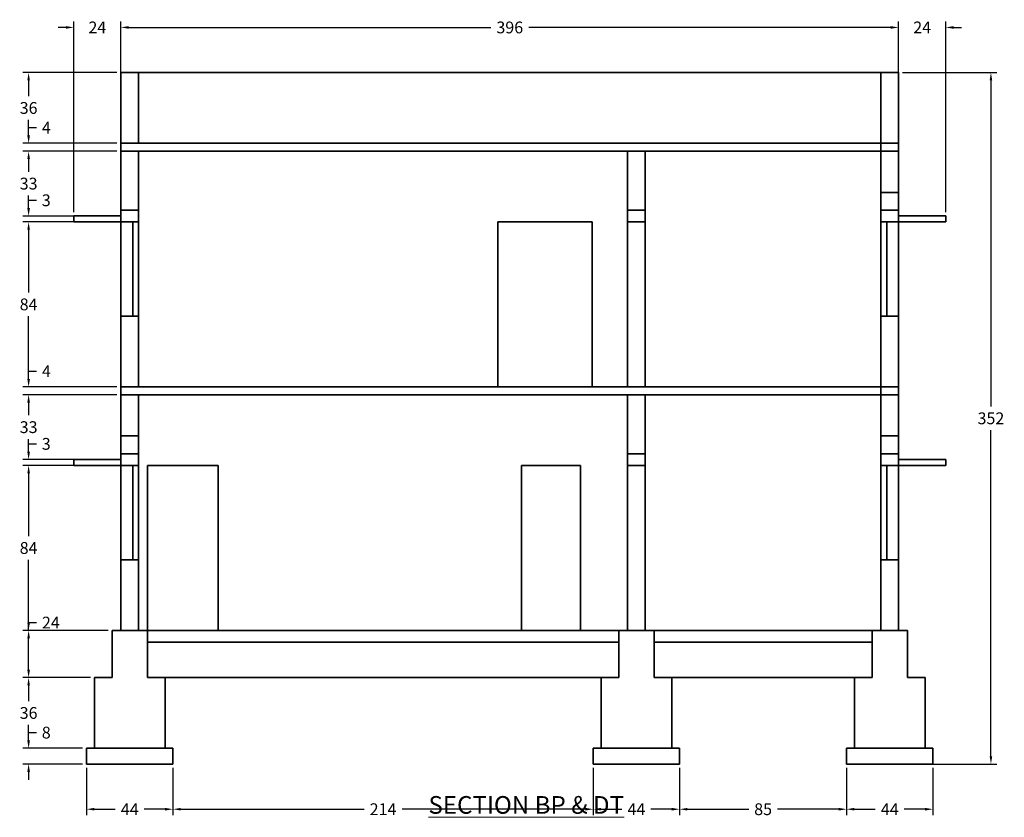
# Model space of a CAD drawing. Units: inches. Extents: x 853 to 2068, y 1026 to 2097.
# Tile 6 of 6: x 1529 to 2030, y 1690 to 2096. Entities that reach past the tile are written whole.
import ezdxf

# ---------------------------------------------------------------- set-up
doc = ezdxf.new("R2010")
doc.units = ezdxf.units.IN
doc.header["$MEASUREMENT"] = 0
for name, color, linetype, lineweight in [('A-ANNO-DIMS', 2, 'Continuous', 18), ('A-ANNO-TEXT', 3, 'Continuous', 18), ('A-SECT', 1, 'Continuous', 35)]:
    doc.layers.add(name, color=color, linetype=linetype, lineweight=lineweight)
doc.styles.get("Standard").update_dxf_attribs({"font": 'arial.ttf'})
doc.dimstyles.get("Standard").update_dxf_attribs({"dimtxt": 6, "dimasz": 4, "dimexe": 3, "dimexo": 2, "dimgap": 3, "dimtad": 0, "dimtih": 1, "dimtoh": 1, "dimdec": 0, "dimzin": 0, "dimdsep": 46, "dimlunit": 3, "dimtxsty": 'Standard', "dimcen": 3, "dimadec": 0, "dimazin": 0, "dimtfac": 1, "dimtdec": 0, "dimtofl": 0, "dimtmove": 0, "dimatfit": 3, "dimfxl": 1, "dimtolj": 1, "dimtzin": 0, "dimarcsym": 0})

# ---------------------------------------------------------------- blocks, each defined once
blk = doc.blocks.new('*D94')
at = {"layer": 'A-ANNO-DIMS', "color": 0, "lineweight": -2, "transparency": 16777216}
for p, q in [((1533.64, 1729.25), (1533.64, 1733.25)), ((1533.64, 1733.25), (1537.64, 1733.25)), ((1561.14, 1725.25), (1530.64, 1725.25)), ((1561.14, 1717.25), (1530.64, 1717.25)), ((1533.64, 1713.25), (1533.64, 1709.25))]:
    blk.add_line(p, q, dxfattribs=at)
at = {"layer": 'A-ANNO-DIMS', "color": 0, "transparency": 16777216}
for points in [[(1532.98, 1729.25), (1534.31, 1729.25), (1533.64, 1725.25)], [(1532.98, 1713.25), (1534.31, 1713.25), (1533.64, 1717.25)]]:
    blk.add_solid(points, dxfattribs=at)
at = {"layer": 'Defpoints', "color": 0, "transparency": 16777216}
for p in [(1533.64, 1725.25), (1563.14, 1725.25), (1563.14, 1717.25)]:
    blk.add_point(p, dxfattribs=at)
at = {"layer": 'A-ANNO-DIMS', "color": 0, "transparency": 16777216, "insert": (1542.62, 1733.25), "char_height": 6, "attachment_point": 5}
blk.add_mtext('\\A1;8', dxfattribs=at)
blk = doc.blocks.new('*D95')
at = {"layer": 'A-ANNO-DIMS', "color": 0, "lineweight": -2, "transparency": 16777216}
for p, q in [((1565.14, 1761.25), (1530.64, 1761.25)), ((1533.64, 1757.25), (1533.64, 1749.32)), ((1533.64, 1729.25), (1533.64, 1737.19)), ((1561.14, 1725.25), (1530.64, 1725.25))]:
    blk.add_line(p, q, dxfattribs=at)
at = {"layer": 'A-ANNO-DIMS', "color": 0, "transparency": 16777216}
for points in [[(1532.98, 1757.25), (1534.31, 1757.25), (1533.64, 1761.25)], [(1532.98, 1729.25), (1534.31, 1729.25), (1533.64, 1725.25)]]:
    blk.add_solid(points, dxfattribs=at)
at = {"layer": 'Defpoints', "color": 0, "transparency": 16777216}
for p in [(1533.64, 1761.25), (1567.14, 1761.25), (1563.14, 1725.25)]:
    blk.add_point(p, dxfattribs=at)
at = {"layer": 'A-ANNO-DIMS', "color": 0, "transparency": 16777216, "insert": (1533.64, 1743.25), "char_height": 6, "attachment_point": 5}
blk.add_mtext('\\A1;36', dxfattribs=at)
blk = doc.blocks.new('*D96')
at = {"layer": 'A-ANNO-DIMS', "color": 0, "lineweight": -2, "transparency": 16777216}
for p, q in [((1574.14, 1785.25), (1530.64, 1785.25)), ((1533.64, 1785.25), (1533.64, 1789.25)), ((1533.64, 1789.25), (1537.64, 1789.25)), ((1533.64, 1765.25), (1533.64, 1781.25)), ((1565.14, 1761.25), (1530.64, 1761.25))]:
    blk.add_line(p, q, dxfattribs=at)
at = {"layer": 'A-ANNO-DIMS', "color": 0, "transparency": 16777216}
for points in [[(1532.98, 1781.25), (1534.31, 1781.25), (1533.64, 1785.25)], [(1532.98, 1765.25), (1534.31, 1765.25), (1533.64, 1761.25)]]:
    blk.add_solid(points, dxfattribs=at)
at = {"layer": 'Defpoints', "color": 0, "transparency": 16777216}
for p in [(1533.64, 1785.25), (1576.14, 1785.25), (1567.14, 1761.25)]:
    blk.add_point(p, dxfattribs=at)
at = {"layer": 'A-ANNO-DIMS', "color": 0, "transparency": 16777216, "insert": (1544.98, 1789.25), "char_height": 6, "attachment_point": 5}
blk.add_mtext('\\A1;24', dxfattribs=at)
blk = doc.blocks.new('*D97')
at = {"layer": 'A-ANNO-DIMS', "color": 0, "lineweight": -2, "transparency": 16777216}
for p, q in [((1578.64, 1869.25), (1530.64, 1869.25)), ((1533.64, 1865.25), (1533.64, 1833.31)), ((1533.64, 1789.25), (1533.64, 1821.19)), ((1574.14, 1785.25), (1530.64, 1785.25))]:
    blk.add_line(p, q, dxfattribs=at)
at = {"layer": 'A-ANNO-DIMS', "color": 0, "transparency": 16777216}
for points in [[(1532.98, 1865.25), (1534.31, 1865.25), (1533.64, 1869.25)], [(1532.98, 1789.25), (1534.31, 1789.25), (1533.64, 1785.25)]]:
    blk.add_solid(points, dxfattribs=at)
at = {"layer": 'Defpoints', "color": 0, "transparency": 16777216}
for p in [(1533.64, 1869.25), (1580.64, 1869.25), (1576.14, 1785.25)]:
    blk.add_point(p, dxfattribs=at)
at = {"layer": 'A-ANNO-DIMS', "color": 0, "transparency": 16777216, "insert": (1533.64, 1827.25), "char_height": 6, "attachment_point": 5}
blk.add_mtext('\\A1;84', dxfattribs=at)
blk = doc.blocks.new('*D98')
at = {"layer": 'A-ANNO-DIMS', "color": 0, "lineweight": -2, "transparency": 16777216}
for p, q in [((1533.64, 1876.25), (1533.64, 1880.25)), ((1533.64, 1880.25), (1537.64, 1880.25)), ((1578.64, 1872.25), (1530.64, 1872.25)), ((1578.64, 1869.25), (1530.64, 1869.25)), ((1533.64, 1865.25), (1533.64, 1861.25))]:
    blk.add_line(p, q, dxfattribs=at)
at = {"layer": 'A-ANNO-DIMS', "color": 0, "transparency": 16777216}
for points in [[(1532.98, 1876.25), (1534.31, 1876.25), (1533.64, 1872.25)], [(1532.98, 1865.25), (1534.31, 1865.25), (1533.64, 1869.25)]]:
    blk.add_solid(points, dxfattribs=at)
at = {"layer": 'Defpoints', "color": 0, "transparency": 16777216}
for p in [(1533.64, 1872.25), (1580.64, 1872.25), (1580.64, 1869.25)]:
    blk.add_point(p, dxfattribs=at)
at = {"layer": 'A-ANNO-DIMS', "color": 0, "transparency": 16777216, "insert": (1542.61, 1880.25), "char_height": 6, "attachment_point": 5}
blk.add_mtext('\\A1;3', dxfattribs=at)
blk = doc.blocks.new('*D99')
at = {"layer": 'A-ANNO-DIMS', "color": 0, "lineweight": -2, "transparency": 16777216}
for p, q in [((1578.64, 1905.25), (1530.64, 1905.25)), ((1533.64, 1901.25), (1533.64, 1894.82)), ((1533.64, 1876.25), (1533.64, 1882.69)), ((1578.64, 1872.25), (1530.64, 1872.25))]:
    blk.add_line(p, q, dxfattribs=at)
at = {"layer": 'A-ANNO-DIMS', "color": 0, "transparency": 16777216}
for points in [[(1532.98, 1901.25), (1534.31, 1901.25), (1533.64, 1905.25)], [(1532.98, 1876.25), (1534.31, 1876.25), (1533.64, 1872.25)]]:
    blk.add_solid(points, dxfattribs=at)
at = {"layer": 'Defpoints', "color": 0, "transparency": 16777216}
for p in [(1533.64, 1905.25), (1580.64, 1905.25), (1580.64, 1872.25)]:
    blk.add_point(p, dxfattribs=at)
at = {"layer": 'A-ANNO-DIMS', "color": 0, "transparency": 16777216, "insert": (1533.64, 1888.75), "char_height": 6, "attachment_point": 5}
blk.add_mtext('\\A1;33', dxfattribs=at)
blk = doc.blocks.new('*D100')
at = {"layer": 'A-ANNO-DIMS', "color": 0, "lineweight": -2, "transparency": 16777216}
for p, q in [((1533.64, 1913.25), (1533.64, 1917.25)), ((1533.64, 1917.25), (1537.64, 1917.25)), ((1578.64, 1909.25), (1530.64, 1909.25)), ((1578.64, 1905.25), (1530.64, 1905.25)), ((1533.64, 1901.25), (1533.64, 1897.25))]:
    blk.add_line(p, q, dxfattribs=at)
at = {"layer": 'A-ANNO-DIMS', "color": 0, "transparency": 16777216}
for points in [[(1532.98, 1913.25), (1534.31, 1913.25), (1533.64, 1909.25)], [(1532.98, 1901.25), (1534.31, 1901.25), (1533.64, 1905.25)]]:
    blk.add_solid(points, dxfattribs=at)
at = {"layer": 'Defpoints', "color": 0, "transparency": 16777216}
for p in [(1533.64, 1909.25), (1580.64, 1909.25), (1580.64, 1905.25)]:
    blk.add_point(p, dxfattribs=at)
at = {"layer": 'A-ANNO-DIMS', "color": 0, "transparency": 16777216, "insert": (1542.72, 1917.25), "char_height": 6, "attachment_point": 5}
blk.add_mtext('\\A1;4', dxfattribs=at)
blk = doc.blocks.new('*D101')
at = {"layer": 'A-ANNO-DIMS', "color": 0, "lineweight": -2, "transparency": 16777216}
for p, q in [((1578.64, 1993.25), (1530.64, 1993.25)), ((1533.64, 1989.25), (1533.64, 1957.31)), ((1533.64, 1913.25), (1533.64, 1945.19)), ((1578.64, 1909.25), (1530.64, 1909.25))]:
    blk.add_line(p, q, dxfattribs=at)
at = {"layer": 'A-ANNO-DIMS', "color": 0, "transparency": 16777216}
for points in [[(1532.98, 1989.25), (1534.31, 1989.25), (1533.64, 1993.25)], [(1532.98, 1913.25), (1534.31, 1913.25), (1533.64, 1909.25)]]:
    blk.add_solid(points, dxfattribs=at)
at = {"layer": 'Defpoints', "color": 0, "transparency": 16777216}
for p in [(1533.64, 1993.25), (1580.64, 1993.25), (1580.64, 1909.25)]:
    blk.add_point(p, dxfattribs=at)
at = {"layer": 'A-ANNO-DIMS', "color": 0, "transparency": 16777216, "insert": (1533.64, 1951.25), "char_height": 6, "attachment_point": 5}
blk.add_mtext('\\A1;84', dxfattribs=at)
blk = doc.blocks.new('*D102')
at = {"layer": 'A-ANNO-DIMS', "color": 0, "lineweight": -2, "transparency": 16777216}
for p, q in [((1533.64, 2000.25), (1533.64, 2004.25)), ((1533.64, 2004.25), (1537.64, 2004.25)), ((1578.64, 1996.25), (1530.64, 1996.25)), ((1578.64, 1993.25), (1530.64, 1993.25)), ((1533.64, 1989.25), (1533.64, 1985.25))]:
    blk.add_line(p, q, dxfattribs=at)
at = {"layer": 'A-ANNO-DIMS', "color": 0, "transparency": 16777216}
for points in [[(1532.98, 2000.25), (1534.31, 2000.25), (1533.64, 1996.25)], [(1532.98, 1989.25), (1534.31, 1989.25), (1533.64, 1993.25)]]:
    blk.add_solid(points, dxfattribs=at)
at = {"layer": 'Defpoints', "color": 0, "transparency": 16777216}
for p in [(1533.64, 1996.25), (1580.64, 1996.25), (1580.64, 1993.25)]:
    blk.add_point(p, dxfattribs=at)
at = {"layer": 'A-ANNO-DIMS', "color": 0, "transparency": 16777216, "insert": (1542.61, 2004.25), "char_height": 6, "attachment_point": 5}
blk.add_mtext('\\A1;3', dxfattribs=at)
blk = doc.blocks.new('*D103')
at = {"layer": 'A-ANNO-DIMS', "color": 0, "lineweight": -2, "transparency": 16777216}
for p, q in [((1578.64, 2029.25), (1530.64, 2029.25)), ((1533.64, 2025.25), (1533.64, 2018.82)), ((1533.64, 2000.25), (1533.64, 2006.69)), ((1578.64, 1996.25), (1530.64, 1996.25))]:
    blk.add_line(p, q, dxfattribs=at)
at = {"layer": 'A-ANNO-DIMS', "color": 0, "transparency": 16777216}
for points in [[(1532.98, 2025.25), (1534.31, 2025.25), (1533.64, 2029.25)], [(1532.98, 2000.25), (1534.31, 2000.25), (1533.64, 1996.25)]]:
    blk.add_solid(points, dxfattribs=at)
at = {"layer": 'Defpoints', "color": 0, "transparency": 16777216}
for p in [(1533.64, 2029.25), (1580.64, 2029.25), (1580.64, 1996.25)]:
    blk.add_point(p, dxfattribs=at)
at = {"layer": 'A-ANNO-DIMS', "color": 0, "transparency": 16777216, "insert": (1533.64, 2012.75), "char_height": 6, "attachment_point": 5}
blk.add_mtext('\\A1;33', dxfattribs=at)
blk = doc.blocks.new('*D104')
at = {"layer": 'A-ANNO-DIMS', "color": 0, "lineweight": -2, "transparency": 16777216}
for p, q in [((1533.64, 2037.25), (1533.64, 2041.25)), ((1533.64, 2041.25), (1537.64, 2041.25)), ((1578.64, 2033.25), (1530.64, 2033.25)), ((1578.64, 2029.25), (1530.64, 2029.25)), ((1533.64, 2025.25), (1533.64, 2021.25))]:
    blk.add_line(p, q, dxfattribs=at)
at = {"layer": 'A-ANNO-DIMS', "color": 0, "transparency": 16777216}
for points in [[(1532.98, 2037.25), (1534.31, 2037.25), (1533.64, 2033.25)], [(1532.98, 2025.25), (1534.31, 2025.25), (1533.64, 2029.25)]]:
    blk.add_solid(points, dxfattribs=at)
at = {"layer": 'Defpoints', "color": 0, "transparency": 16777216}
for p in [(1533.64, 2033.25), (1580.64, 2033.25), (1580.64, 2029.25)]:
    blk.add_point(p, dxfattribs=at)
at = {"layer": 'A-ANNO-DIMS', "color": 0, "transparency": 16777216, "insert": (1542.72, 2041.25), "char_height": 6, "attachment_point": 5}
blk.add_mtext('\\A1;4', dxfattribs=at)
blk = doc.blocks.new('*D105')
at = {"layer": 'A-ANNO-DIMS', "color": 0, "lineweight": -2, "transparency": 16777216}
for p, q in [((1578.64, 2069.25), (1530.64, 2069.25)), ((1533.64, 2065.25), (1533.64, 2057.32)), ((1533.64, 2037.25), (1533.64, 2045.19)), ((1578.64, 2033.25), (1530.64, 2033.25))]:
    blk.add_line(p, q, dxfattribs=at)
at = {"layer": 'A-ANNO-DIMS', "color": 0, "transparency": 16777216}
for points in [[(1532.98, 2065.25), (1534.31, 2065.25), (1533.64, 2069.25)], [(1532.98, 2037.25), (1534.31, 2037.25), (1533.64, 2033.25)]]:
    blk.add_solid(points, dxfattribs=at)
at = {"layer": 'Defpoints', "color": 0, "transparency": 16777216}
for p in [(1533.64, 2069.25), (1580.64, 2069.25), (1580.64, 2033.25)]:
    blk.add_point(p, dxfattribs=at)
at = {"layer": 'A-ANNO-DIMS', "color": 0, "transparency": 16777216, "insert": (1533.64, 2051.25), "char_height": 6, "attachment_point": 5}
blk.add_mtext('\\A1;36', dxfattribs=at)
blk = doc.blocks.new('*D106')
at = {"layer": 'A-ANNO-DIMS', "color": 0, "lineweight": -2, "transparency": 16777216}
for p, q in [((1978.64, 2069.25), (2026.64, 2069.25)), ((2023.64, 2065.25), (2023.64, 1899.32)), ((2023.64, 1721.25), (2023.64, 1887.19)), ((1969.64, 1717.25), (2026.64, 1717.25))]:
    blk.add_line(p, q, dxfattribs=at)
at = {"layer": 'A-ANNO-DIMS', "color": 0, "transparency": 16777216}
for points in [[(2022.98, 2065.25), (2024.31, 2065.25), (2023.64, 2069.25)], [(2022.98, 1721.25), (2024.31, 1721.25), (2023.64, 1717.25)]]:
    blk.add_solid(points, dxfattribs=at)
at = {"layer": 'Defpoints', "color": 0, "transparency": 16777216}
for p in [(1976.64, 2069.25), (2023.64, 2069.25), (1967.64, 1717.25)]:
    blk.add_point(p, dxfattribs=at)
at = {"layer": 'A-ANNO-DIMS', "color": 0, "transparency": 16777216, "insert": (2023.64, 1893.25), "char_height": 6, "attachment_point": 5}
blk.add_mtext('\\A1;352', dxfattribs=at)
blk = doc.blocks.new('*D107')
at = {"layer": 'A-ANNO-DIMS', "color": 0, "lineweight": -2, "transparency": 16777216}
for p, q in [((1563.14, 1715.25), (1563.14, 1691.25)), ((1607.14, 1715.25), (1607.14, 1691.25)), ((1567.14, 1694.25), (1577.74, 1694.25)), ((1603.14, 1694.25), (1592.55, 1694.25))]:
    blk.add_line(p, q, dxfattribs=at)
at = {"layer": 'A-ANNO-DIMS', "color": 0, "transparency": 16777216}
for points in [[(1567.14, 1694.92), (1567.14, 1693.58), (1563.14, 1694.25)], [(1603.14, 1694.92), (1603.14, 1693.58), (1607.14, 1694.25)]]:
    blk.add_solid(points, dxfattribs=at)
at = {"layer": 'Defpoints', "color": 0, "transparency": 16777216}
for p in [(1563.14, 1717.25), (1607.14, 1717.25), (1607.14, 1694.25)]:
    blk.add_point(p, dxfattribs=at)
at = {"layer": 'A-ANNO-DIMS', "color": 0, "transparency": 16777216, "insert": (1585.14, 1694.25), "char_height": 6, "attachment_point": 5}
blk.add_mtext('\\A1;44', dxfattribs=at)
blk = doc.blocks.new('*D108')
at = {"layer": 'A-ANNO-DIMS', "color": 0, "lineweight": -2, "transparency": 16777216}
for p, q in [((1607.14, 1715.25), (1607.14, 1691.25)), ((1821.14, 1715.25), (1821.14, 1691.25)), ((1611.14, 1694.25), (1704.47, 1694.25)), ((1817.14, 1694.25), (1723.81, 1694.25))]:
    blk.add_line(p, q, dxfattribs=at)
at = {"layer": 'A-ANNO-DIMS', "color": 0, "transparency": 16777216}
for points in [[(1611.14, 1694.92), (1611.14, 1693.58), (1607.14, 1694.25)], [(1817.14, 1694.92), (1817.14, 1693.58), (1821.14, 1694.25)]]:
    blk.add_solid(points, dxfattribs=at)
at = {"layer": 'Defpoints', "color": 0, "transparency": 16777216}
for p in [(1607.14, 1717.25), (1821.14, 1717.25), (1821.14, 1694.25)]:
    blk.add_point(p, dxfattribs=at)
at = {"layer": 'A-ANNO-DIMS', "color": 0, "transparency": 16777216, "insert": (1714.14, 1694.25), "char_height": 6, "attachment_point": 5}
blk.add_mtext('\\A1;214', dxfattribs=at)
blk = doc.blocks.new('*D109')
at = {"layer": 'A-ANNO-DIMS', "color": 0, "lineweight": -2, "transparency": 16777216}
for p, q in [((1821.14, 1715.25), (1821.14, 1691.25)), ((1865.14, 1715.25), (1865.14, 1691.25)), ((1825.14, 1694.25), (1835.74, 1694.25)), ((1861.14, 1694.25), (1850.55, 1694.25))]:
    blk.add_line(p, q, dxfattribs=at)
at = {"layer": 'A-ANNO-DIMS', "color": 0, "transparency": 16777216}
for points in [[(1825.14, 1694.92), (1825.14, 1693.58), (1821.14, 1694.25)], [(1861.14, 1694.92), (1861.14, 1693.58), (1865.14, 1694.25)]]:
    blk.add_solid(points, dxfattribs=at)
at = {"layer": 'Defpoints', "color": 0, "transparency": 16777216}
for p in [(1821.14, 1717.25), (1865.14, 1717.25), (1865.14, 1694.25)]:
    blk.add_point(p, dxfattribs=at)
at = {"layer": 'A-ANNO-DIMS', "color": 0, "transparency": 16777216, "insert": (1843.14, 1694.25), "char_height": 6, "attachment_point": 5}
blk.add_mtext('\\A1;44', dxfattribs=at)
blk = doc.blocks.new('*D110')
at = {"layer": 'A-ANNO-DIMS', "color": 0, "lineweight": -2, "transparency": 16777216}
for p, q in [((1865.14, 1715.25), (1865.14, 1691.25)), ((1950.14, 1715.25), (1950.14, 1691.25)), ((1869.14, 1694.25), (1900.32, 1694.25)), ((1946.14, 1694.25), (1914.97, 1694.25))]:
    blk.add_line(p, q, dxfattribs=at)
at = {"layer": 'A-ANNO-DIMS', "color": 0, "transparency": 16777216}
for points in [[(1869.14, 1694.92), (1869.14, 1693.58), (1865.14, 1694.25)], [(1946.14, 1694.92), (1946.14, 1693.58), (1950.14, 1694.25)]]:
    blk.add_solid(points, dxfattribs=at)
at = {"layer": 'Defpoints', "color": 0, "transparency": 16777216}
for p in [(1865.14, 1717.25), (1950.14, 1717.25), (1950.14, 1694.25)]:
    blk.add_point(p, dxfattribs=at)
at = {"layer": 'A-ANNO-DIMS', "color": 0, "transparency": 16777216, "insert": (1907.64, 1694.25), "char_height": 6, "attachment_point": 5}
blk.add_mtext('\\A1;85', dxfattribs=at)
blk = doc.blocks.new('*D111')
at = {"layer": 'A-ANNO-DIMS', "color": 0, "lineweight": -2, "transparency": 16777216}
for p, q in [((1950.14, 1715.25), (1950.14, 1691.25)), ((1994.14, 1715.25), (1994.14, 1691.25)), ((1954.14, 1694.25), (1964.74, 1694.25)), ((1990.14, 1694.25), (1979.55, 1694.25))]:
    blk.add_line(p, q, dxfattribs=at)
at = {"layer": 'A-ANNO-DIMS', "color": 0, "transparency": 16777216}
for points in [[(1954.14, 1694.92), (1954.14, 1693.58), (1950.14, 1694.25)], [(1990.14, 1694.92), (1990.14, 1693.58), (1994.14, 1694.25)]]:
    blk.add_solid(points, dxfattribs=at)
at = {"layer": 'Defpoints', "color": 0, "transparency": 16777216}
for p in [(1950.14, 1717.25), (1994.14, 1717.25), (1994.14, 1694.25)]:
    blk.add_point(p, dxfattribs=at)
at = {"layer": 'A-ANNO-DIMS', "color": 0, "transparency": 16777216, "insert": (1972.14, 1694.25), "char_height": 6, "attachment_point": 5}
blk.add_mtext('\\A1;44', dxfattribs=at)
blk = doc.blocks.new('*D112')
at = {"layer": 'A-ANNO-DIMS', "color": 0, "lineweight": -2, "transparency": 16777216}
for p, q in [((1552.64, 2092.25), (1548.64, 2092.25)), ((1556.64, 1998.25), (1556.64, 2095.25)), ((1580.64, 1998.25), (1580.64, 2095.25)), ((1584.64, 2092.25), (1588.64, 2092.25))]:
    blk.add_line(p, q, dxfattribs=at)
at = {"layer": 'A-ANNO-DIMS', "color": 0, "transparency": 16777216}
for points in [[(1552.64, 2092.92), (1552.64, 2091.58), (1556.64, 2092.25)], [(1584.64, 2092.92), (1584.64, 2091.58), (1580.64, 2092.25)]]:
    blk.add_solid(points, dxfattribs=at)
at = {"layer": 'Defpoints', "color": 0, "transparency": 16777216}
for p in [(1580.64, 2092.25), (1556.64, 1996.25), (1580.64, 1996.25)]:
    blk.add_point(p, dxfattribs=at)
at = {"layer": 'A-ANNO-DIMS', "color": 0, "transparency": 16777216, "insert": (1568.64, 2092.25), "char_height": 6, "attachment_point": 5}
blk.add_mtext('\\A1;24', dxfattribs=at)
blk = doc.blocks.new('*D113')
at = {"layer": 'A-ANNO-DIMS', "color": 0, "lineweight": -2, "transparency": 16777216}
for p, q in [((1580.64, 2071.25), (1580.64, 2095.25)), ((1584.64, 2092.25), (1769.02, 2092.25)), ((1972.64, 2092.25), (1788.27, 2092.25)), ((1976.64, 2071.25), (1976.64, 2095.25))]:
    blk.add_line(p, q, dxfattribs=at)
at = {"layer": 'A-ANNO-DIMS', "color": 0, "transparency": 16777216}
for points in [[(1584.64, 2092.92), (1584.64, 2091.58), (1580.64, 2092.25)], [(1972.64, 2092.92), (1972.64, 2091.58), (1976.64, 2092.25)]]:
    blk.add_solid(points, dxfattribs=at)
at = {"layer": 'Defpoints', "color": 0, "transparency": 16777216}
for p in [(1976.64, 2092.25), (1580.64, 2069.25), (1976.64, 2069.25)]:
    blk.add_point(p, dxfattribs=at)
at = {"layer": 'A-ANNO-DIMS', "color": 0, "transparency": 16777216, "insert": (1778.64, 2092.25), "char_height": 6, "attachment_point": 5}
blk.add_mtext('\\A1;396', dxfattribs=at)
blk = doc.blocks.new('*D114')
at = {"layer": 'A-ANNO-DIMS', "color": 0, "lineweight": -2, "transparency": 16777216}
for p, q in [((1972.64, 2092.25), (1968.64, 2092.25)), ((1976.64, 1998.25), (1976.64, 2095.25)), ((2000.64, 1998.25), (2000.64, 2095.25)), ((2004.64, 2092.25), (2008.64, 2092.25))]:
    blk.add_line(p, q, dxfattribs=at)
at = {"layer": 'A-ANNO-DIMS', "color": 0, "transparency": 16777216}
for points in [[(1972.64, 2092.92), (1972.64, 2091.58), (1976.64, 2092.25)], [(2004.64, 2092.92), (2004.64, 2091.58), (2000.64, 2092.25)]]:
    blk.add_solid(points, dxfattribs=at)
at = {"layer": 'Defpoints', "color": 0, "transparency": 16777216}
for p in [(2000.64, 2092.25), (1976.64, 1996.25), (2000.64, 1996.25)]:
    blk.add_point(p, dxfattribs=at)
at = {"layer": 'A-ANNO-DIMS', "color": 0, "transparency": 16777216, "insert": (1988.64, 2092.25), "char_height": 6, "attachment_point": 5}
blk.add_mtext('\\A1;24', dxfattribs=at)

msp = doc.modelspace()

# ---------------------------------------------------------------- linework, layer by layer
at = {"layer": 'A-SECT'}
for p, q in [((1580.642, 2069.2513), (1976.642, 2069.2513)), ((1580.642, 1785.2513), (1580.642, 2069.2513)), ((1589.642, 2033.2513), (1589.642, 2069.2513)), ((1967.642, 1785.2513), (1967.642, 2069.2513)), ((1976.642, 1785.2513), (1976.642, 2069.2513)), ((1580.642, 2033.2513), (1976.642, 2033.2513)), ((1580.642, 2029.2513), (1976.642, 2029.2513)), ((1589.642, 1909.2513), (1589.642, 2029.2513)), ((1838.642, 1909.2513), (1838.642, 2029.2513)), ((1847.642, 1909.2513), (1847.642, 2029.2513)), ((1976.642, 2008.2513), (1967.642, 2008.2513)), ((1556.642, 1993.2513), (1556.642, 1996.2513)), ((1556.642, 1996.2513), (1580.642, 1996.2513)), ((1580.642, 1996.2513), (1580.642, 1999.2513)), ((1580.642, 1999.2513), (1589.642, 1999.2513)), ((1838.642, 1999.2513), (1847.642, 1999.2513)), ((1976.642, 1999.2513), (1967.642, 1999.2513)), ((1976.642, 1996.2513), (1976.642, 1999.2513)), ((2000.642, 1996.2513), (1976.642, 1996.2513)), ((2000.642, 1993.2513), (2000.642, 1996.2513)), ((1580.642, 1993.2513), (1556.642, 1993.2513)), ((1589.642, 1993.2513), (1580.642, 1993.2513)), ((1586.642, 1993.2513), (1586.642, 1945.2513)), ((1772.642, 1909.2513), (1772.642, 1993.2513)), ((1820.642, 1993.2513), (1772.642, 1993.2513)), ((1820.642, 1909.2513), (1820.642, 1993.2513)), ((1838.642, 1993.2513), (1847.642, 1993.2513)), ((1967.642, 1993.2513), (1976.642, 1993.2513)), ((1970.642, 1993.2513), (1970.642, 1945.2513)), ((1976.642, 1993.2513), (2000.642, 1993.2513)), ((1589.642, 1945.2513), (1580.642, 1945.2513)), ((1589.642, 1945.2513), (1580.642, 1945.2513)), ((1967.642, 1945.2513), (1976.642, 1945.2513)), ((1580.642, 1909.2513), (1976.642, 1909.2513)), ((1580.642, 1905.2513), (1976.642, 1905.2513)), ((1589.642, 1785.2513), (1589.642, 1905.2513)), ((1838.642, 1785.2513), (1838.642, 1905.2513)), ((1847.642, 1785.2513), (1847.642, 1905.2513)), ((1580.642, 1884.2513), (1589.642, 1884.2513)), ((1976.642, 1884.2513), (1967.642, 1884.2513)), ((1580.642, 1872.2513), (1580.642, 1875.2513)), ((1580.642, 1875.2513), (1589.642, 1875.2513)), ((1838.642, 1875.2513), (1847.642, 1875.2513)), ((1976.642, 1875.2513), (1967.642, 1875.2513)), ((1976.642, 1872.2513), (1976.642, 1875.2513)), ((1556.642, 1869.2513), (1556.642, 1872.2513)), ((1556.642, 1872.2513), (1580.642, 1872.2513)), ((2000.642, 1872.2513), (1976.642, 1872.2513)), ((2000.642, 1869.2513), (2000.642, 1872.2513)), ((1580.642, 1869.2513), (1556.642, 1869.2513)), ((1589.642, 1869.2513), (1580.642, 1869.2513)), ((1586.642, 1869.2513), (1586.642, 1821.2513)), ((1594.142, 1785.2513), (1594.142, 1869.2513)), ((1594.142, 1869.2513), (1630.142, 1869.2513)), ((1630.142, 1869.2513), (1630.142, 1785.2513)), ((1784.642, 1785.2513), (1784.642, 1869.2513)), ((1814.642, 1869.2513), (1784.642, 1869.2513)), ((1814.642, 1785.2513), (1814.642, 1869.2513)), ((1838.642, 1869.2513), (1847.642, 1869.2513)), ((1967.642, 1869.2513), (1976.642, 1869.2513)), ((1970.642, 1869.2513), (1970.642, 1821.2513)), ((1976.642, 1869.2513), (2000.642, 1869.2513)), ((1589.642, 1821.2513), (1580.642, 1821.2513)), ((1967.642, 1821.2513), (1976.642, 1821.2513)), ((1576.142, 1785.2513), (1976.642, 1785.2513)), ((1585.142, 1785.2513), (1576.142, 1785.2513)), ((1576.142, 1785.2513), (1576.142, 1761.2513)), ((1585.142, 1785.2513), (1585.142, 1785.2513)), ((1585.142, 1785.2513), (1594.142, 1785.2513)), ((1594.142, 1785.2513), (1594.142, 1761.2513)), ((1843.142, 1785.2513), (1834.142, 1785.2513)), ((1834.142, 1785.2513), (1834.142, 1761.2513)), ((1843.142, 1785.2513), (1852.142, 1785.2513)), ((1852.142, 1785.2513), (1852.142, 1761.2513)), ((1972.142, 1785.2513), (1963.142, 1785.2513)), ((1963.142, 1785.2513), (1963.142, 1761.2513)), ((1972.142, 1785.2513), (1981.142, 1785.2513)), ((1981.142, 1785.2513), (1981.142, 1761.2513)), ((1594.142, 1779.2513), (1834.142, 1779.2513)), ((1852.142, 1779.2513), (1963.142, 1779.2513)), ((1576.142, 1761.2513), (1567.142, 1761.2513)), ((1567.142, 1761.2513), (1567.142, 1725.2513)), ((1594.142, 1761.2513), (1603.142, 1761.2513)), ((1603.142, 1761.2513), (1603.142, 1725.2513)), ((1603.142, 1761.2513), (1825.142, 1761.2513)), ((1834.142, 1761.2513), (1825.142, 1761.2513)), ((1825.142, 1761.2513), (1825.142, 1725.2513)), ((1852.142, 1761.2513), (1861.142, 1761.2513)), ((1861.142, 1761.2513), (1861.142, 1725.2513)), ((1861.142, 1761.2513), (1954.142, 1761.2513)), ((1963.142, 1761.2513), (1954.142, 1761.2513)), ((1954.142, 1761.2513), (1954.142, 1725.2513)), ((1981.142, 1761.2513), (1990.142, 1761.2513)), ((1990.142, 1761.2513), (1990.142, 1725.2513)), ((1567.142, 1725.2513), (1563.142, 1725.2513)), ((1563.142, 1725.2513), (1563.142, 1717.2513)), ((1567.142, 1725.2513), (1607.142, 1725.2513)), ((1603.142, 1725.2513), (1607.142, 1725.2513)), ((1607.142, 1725.2513), (1607.142, 1717.2513)), ((1825.142, 1725.2513), (1821.142, 1725.2513)), ((1821.142, 1725.2513), (1821.142, 1717.2513)), ((1825.142, 1725.2513), (1865.142, 1725.2513)), ((1861.142, 1725.2513), (1865.142, 1725.2513)), ((1865.142, 1725.2513), (1865.142, 1717.2513)), ((1954.142, 1725.2513), (1950.142, 1725.2513)), ((1950.142, 1725.2513), (1950.142, 1717.2513)), ((1954.142, 1725.2513), (1994.142, 1725.2513)), ((1990.142, 1725.2513), (1994.142, 1725.2513)), ((1994.142, 1725.2513), (1994.142, 1717.2513)), ((1563.142, 1717.2513), (1607.142, 1717.2513)), ((1580.642, 1717.2513), (1607.142, 1717.2513)), ((1821.142, 1717.2513), (1865.142, 1717.2513)), ((1838.642, 1717.2513), (1865.142, 1717.2513)), ((1950.142, 1717.2513), (1994.142, 1717.2513)), ((1967.642, 1717.2513), (1994.142, 1717.2513))]:
    msp.add_line(p, q, dxfattribs=at)

# ---------------------------------------------------------------- texts
at = {"layer": 'A-ANNO-TEXT', "insert": (1737.244, 1700.9302), "char_height": 9, "attachment_point": 1}
msp.add_mtext_dynamic_manual_height_columns('{\\LSECTION BP & DT}', width=227.402365, gutter_width=1, heights=[0], dxfattribs=at)

# ---------------------------------------------------------------- dimensions: what is measured, and where the dimension line sits
at = {"layer": 'A-ANNO-DIMS'}
for base, p1, p2, picture, middle in [((1580.642, 2092.2513), (1556.642, 1996.2513), (1580.642, 1996.2513), '*D112', (1568.642, 2092.2513)), ((1976.642, 2092.2513), (1580.642, 2069.2513), (1976.642, 2069.2513), '*D113', (1778.642, 2092.2513)), ((2000.642, 2092.2513), (1976.642, 1996.2513), (2000.642, 1996.2513), '*D114', (1988.642, 2092.2513)), ((1607.142, 1694.2513), (1563.142, 1717.2513), (1607.142, 1717.2513), '*D107', (1585.142, 1694.2513)), ((1821.142, 1694.2513), (1607.142, 1717.2513), (1821.142, 1717.2513), '*D108', (1714.142, 1694.2513)), ((1865.142, 1694.2513), (1821.142, 1717.2513), (1865.142, 1717.2513), '*D109', (1843.142, 1694.2513)), ((1950.142, 1694.2513), (1865.142, 1717.2513), (1950.142, 1717.2513), '*D110', (1907.642, 1694.2513)), ((1994.142, 1694.2513), (1950.142, 1717.2513), (1994.142, 1717.2513), '*D111', (1972.142, 1694.2513))]:
    dim = msp.add_linear_dim(base=base, p1=p1, p2=p2, dimstyle='Standard', override={"dimdec": 0, "dimlfac": 1, "dimrnd": 0, "dimzin": 0, "dimdsep": 46, "dimlunit": 2}, dxfattribs=at)
    dim.commit()
    dim.dimension.update_dxf_attribs({"geometry": picture, "text_midpoint": middle})
for base, p1, p2, picture, middle in [((1533.642, 2069.2513), (1580.642, 2033.2513), (1580.642, 2069.2513), '*D105', (1533.642, 2051.2513)), ((2023.642, 2069.2513), (1967.642, 1717.2513), (1976.642, 2069.2513), '*D106', (2023.642, 1893.2513)), ((1533.642, 2033.2513), (1580.642, 2029.2513), (1580.642, 2033.2513), '*D104', (1542.7171, 2041.2513)), ((1533.642, 2029.2513), (1580.642, 1996.2513), (1580.642, 2029.2513), '*D103', (1533.642, 2012.7513)), ((1533.642, 1996.2513), (1580.642, 1993.2513), (1580.642, 1996.2513), '*D102', (1542.6066, 2004.2513)), ((1533.642, 1993.2513), (1580.642, 1909.2513), (1580.642, 1993.2513), '*D101', (1533.642, 1951.2513)), ((1533.642, 1909.2513), (1580.642, 1905.2513), (1580.642, 1909.2513), '*D100', (1542.7171, 1917.2513)), ((1533.642, 1905.2513), (1580.642, 1872.2513), (1580.642, 1905.2513), '*D99', (1533.642, 1888.7513)), ((1533.642, 1872.2513), (1580.642, 1869.2513), (1580.642, 1872.2513), '*D98', (1542.6066, 1880.2513)), ((1533.642, 1869.2513), (1576.142, 1785.2513), (1580.642, 1869.2513), '*D97', (1533.642, 1827.2513)), ((1533.642, 1785.2513), (1567.142, 1761.2513), (1576.142, 1785.2513), '*D96', (1544.9783, 1789.2513)), ((1533.642, 1761.2513), (1563.142, 1725.2513), (1567.142, 1761.2513), '*D95', (1533.642, 1743.2513)), ((1533.642, 1725.2513), (1563.142, 1717.2513), (1563.142, 1725.2513), '*D94', (1542.6188, 1733.2513))]:
    dim = msp.add_linear_dim(base=base, p1=p1, p2=p2, angle=90, dimstyle='Standard', override={"dimdec": 0, "dimlfac": 1, "dimrnd": 0, "dimzin": 0, "dimdsep": 46, "dimlunit": 2}, dxfattribs=at)
    dim.commit()
    dim.dimension.update_dxf_attribs({"geometry": picture, "text_midpoint": middle})

doc.saveas('drawing.dxf')
